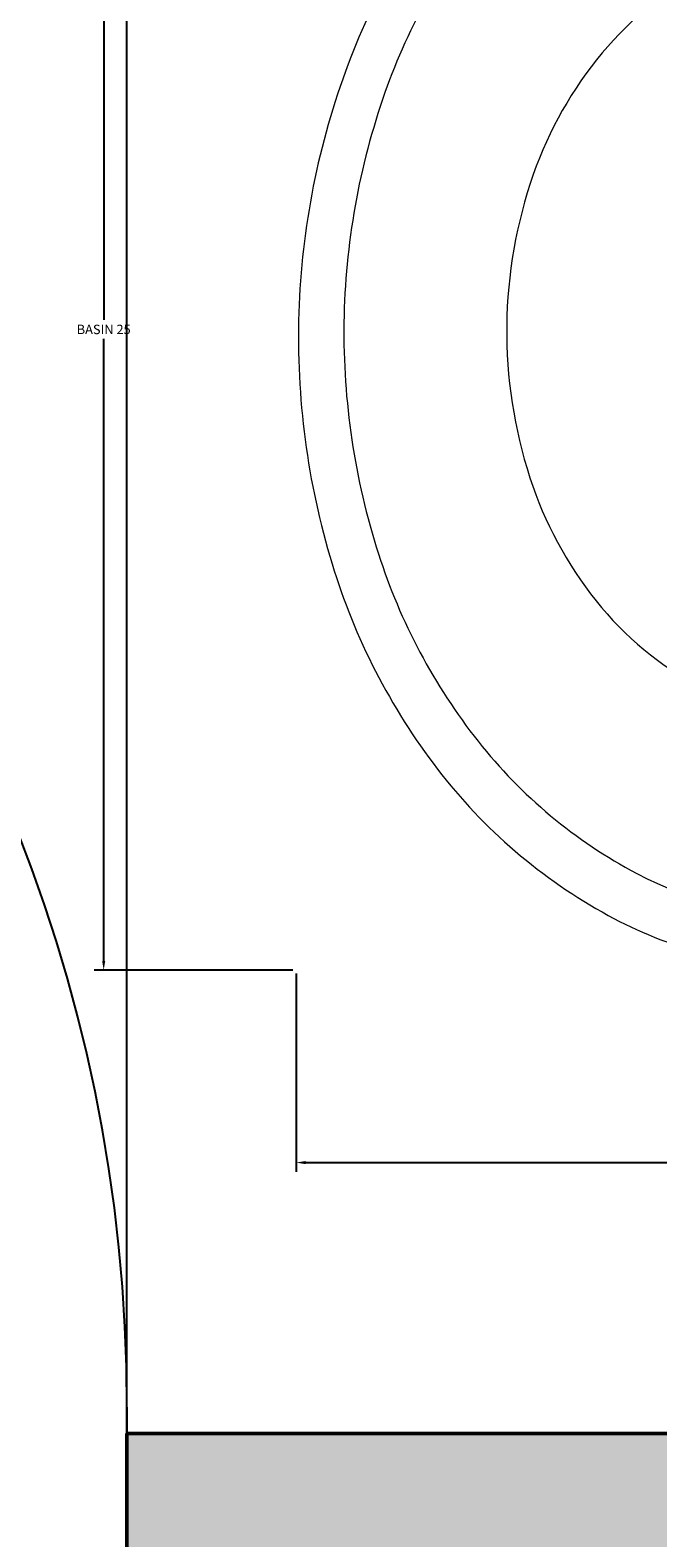
# Model space of a CAD drawing. Units: inches. Extents: x 2307 to 2544, y 2171 to 2540.
# Tile 41 of 52: x 2490 to 2502, y 2438 to 2466. Entities that reach past the tile are written whole.
import ezdxf

# ---------------------------------------------------------------- set-up
doc = ezdxf.new("R2010")
doc.units = ezdxf.units.IN
for name, color, linetype, lineweight in [('A-ANNO-DIMS', 2, 'Continuous', 18), ('A-DOOR', 3, 'Continuous', 25), ('A-FLOR-FIXT', 9, 'Continuous', 18), ('A-WALL', 7, 'Continuous', 50)]:
    doc.layers.add(name, color=color, linetype=linetype, lineweight=lineweight)
doc.layers.add('A-WALL-PATT', color=18, linetype='Continuous', lineweight=13, true_color=0x000000)
doc.styles.get("Standard").update_dxf_attribs({"font": 'arial.ttf'})
doc.dimstyles.get("Standard").update_dxf_attribs({"dimtxt": 0.18, "dimasz": 0.18, "dimexe": 0.18, "dimexo": 0.0625, "dimgap": 0.09, "dimtad": 0, "dimtih": 1, "dimtoh": 1, "dimdec": 4, "dimzin": 0, "dimdsep": 46, "dimtxsty": 'Standard', "dimcen": 0.09, "dimadec": 0, "dimazin": 0, "dimtfac": 1, "dimtdec": 4, "dimtofl": 0, "dimtmove": 0, "dimatfit": 3, "dimfxl": 1, "dimtolj": 1, "dimtzin": 0, "dimarcsym": 0})

# ---------------------------------------------------------------- blocks, each defined once
blk = doc.blocks.new('Sink - Oval top')
for p, q in [((0, 1), (0, -1)), ((-1, 0), (1, 0))]:
    blk.add_line(p, q)
for points in [[(-12.234, 0.394, 0.117634), (-11.465, -3.362, 0.104469), (-8.879, -6.804, 0.090016), (-5.083, -9.072, 0.08192), (-0.323, -10.016, 0.08192), (4.488, -9.381, 0.090016), (8.422, -7.361, 0.104469), (11.224, -4.093, 0.117634), (12.234, -0.394, 0.117634), (11.465, 3.362, 0.104469), (8.879, 6.804, 0.090016), (5.083, 9.072, 0.08192), (0.323, 10.016, 0.08192), (-4.488, 9.381, 0.090016), (-8.422, 7.361, 0.104469), (-11.224, 4.093, 0.117634)], [(-11.286, 0.159, 0.118622), (-10.516, -3.253, 0.104678), (-8.072, -6.359, 0.089562), (-4.538, -8.367, 0.081185), (-0.129, -9.152, 0.081185), (4.3, -8.492, 0.089562), (7.889, -6.584, 0.104678), (10.42, -3.548, 0.118622), (11.286, -0.159, 0.118622), (10.516, 3.253, 0.104678), (8.072, 6.359, 0.089562), (4.538, 8.367, 0.081185), (0.129, 9.152, 0.081185), (-4.3, 8.492, 0.089562), (-7.889, 6.584, 0.104678), (-10.42, 3.548, 0.118622)], [(-7.42, 0.083, 0.118283), (-6.907, -2.167, 0.104607), (-5.295, -4.21, 0.089718), (-2.967, -5.528, 0.081436), (-0.068, -6.037, 0.081436), (2.842, -5.593, 0.089718), (5.199, -4.327, 0.104607), (6.857, -2.321, 0.118283), (7.42, -0.083, 0.118283), (6.907, 2.167, 0.104607), (5.295, 4.21, 0.089718), (2.967, 5.528, 0.081436), (0.068, 6.037, 0.081436), (-2.842, 5.593, 0.089718), (-5.199, 4.327, 0.104607), (-6.857, 2.321, 0.118283)]]:
    blk.add_lwpolyline(points, format="xyb", close=True)
for radius in [1.5, 1]:
    blk.add_circle((0, 0), radius)
blk = doc.blocks.new('*U13')
blk.add_line((40, 0), (40, -6))
blk.add_arc((0, 0), 40, 0, 90)
blk = doc.blocks.new('*D22')
at = {"layer": 'A-ANNO-DIMS', "color": 0, "lineweight": -2, "transparency": 16777216}
for p, q in [((2494.871, 2472.93), (2491.071, 2472.93)), ((2491.251, 2472.75), (2491.251, 2460.838)), ((2491.251, 2448.56), (2491.251, 2460.472)), ((2494.871, 2448.38), (2491.071, 2448.38))]:
    blk.add_line(p, q, dxfattribs=at)
at = {"layer": 'A-ANNO-DIMS', "color": 0, "transparency": 16777216}
for points in [[(2491.221, 2472.75), (2491.281, 2472.75), (2491.251, 2472.93)], [(2491.221, 2448.56), (2491.281, 2448.56), (2491.251, 2448.38)]]:
    blk.add_solid(points, dxfattribs=at)
at = {"layer": 'Defpoints', "color": 0, "transparency": 16777216}
for p in [(2494.934, 2472.93), (2491.251, 2448.38), (2494.934, 2448.38)]:
    blk.add_point(p, dxfattribs=at)
at = {"layer": 'A-ANNO-DIMS', "color": 0, "transparency": 16777216, "insert": (2491.251, 2460.655), "char_height": 0.18, "attachment_point": 5}
blk.add_mtext('\\A1;BASIN 25', dxfattribs=at)
blk = doc.blocks.new('*D23')
at = {"layer": 'A-ANNO-DIMS', "color": 0, "lineweight": -2, "transparency": 16777216}
for p, q in [((2494.934, 2448.317), (2494.934, 2444.517)), ((2515.07, 2448.317), (2515.07, 2444.517)), ((2495.114, 2444.697), (2504.782, 2444.697)), ((2514.89, 2444.697), (2505.222, 2444.697))]:
    blk.add_line(p, q, dxfattribs=at)
at = {"layer": 'A-ANNO-DIMS', "color": 0, "transparency": 16777216}
for points in [[(2495.114, 2444.727), (2495.114, 2444.667), (2494.934, 2444.697)], [(2514.89, 2444.727), (2514.89, 2444.667), (2515.07, 2444.697)]]:
    blk.add_solid(points, dxfattribs=at)
at = {"layer": 'Defpoints', "color": 0, "transparency": 16777216}
for p in [(2494.934, 2448.38), (2515.07, 2448.38), (2515.07, 2444.697)]:
    blk.add_point(p, dxfattribs=at)
at = {"layer": 'A-ANNO-DIMS', "color": 0, "transparency": 16777216, "insert": (2505.002, 2444.697), "char_height": 0.18, "attachment_point": 5}
blk.add_mtext('\\A1;20', dxfattribs=at)
blk = doc.blocks.new('*D61')
at = {"layer": 'A-ANNO-DIMS', "color": 0, "lineweight": -2, "transparency": 16777216}
for p, q in [((2491.696, 2435.572), (2491.696, 2540.345)), ((2515.696, 2435.572), (2515.696, 2540.345)), ((2491.876, 2540.165), (2503.476, 2540.165)), ((2515.516, 2540.165), (2503.916, 2540.165))]:
    blk.add_line(p, q, dxfattribs=at)
at = {"layer": 'A-ANNO-DIMS', "color": 0, "transparency": 16777216}
for points in [[(2491.876, 2540.195), (2491.876, 2540.135), (2491.696, 2540.165)], [(2515.516, 2540.195), (2515.516, 2540.135), (2515.696, 2540.165)]]:
    blk.add_solid(points, dxfattribs=at)
at = {"layer": 'Defpoints', "color": 0, "transparency": 16777216}
for p in [(2515.696, 2540.165), (2491.696, 2435.51), (2515.696, 2435.51)]:
    blk.add_point(p, dxfattribs=at)
at = {"layer": 'A-ANNO-DIMS', "color": 0, "transparency": 16777216, "insert": (2503.696, 2540.165), "char_height": 0.18, "attachment_point": 5}
blk.add_mtext('\\A1;24', dxfattribs=at)

msp = doc.modelspace()

# ---------------------------------------------------------------- hatches: boundary and pattern name
at = {"layer": 'A-WALL-PATT'}
h = msp.add_hatch(color=256, dxfattribs=at)
h.dxf.hatch_style = 1
h.paths.add_polyline_path([(2433.6935, 2199.5096), (2415.6423, 2199.5096), (2415.6423, 2190.5096), (2433.7832, 2190.5096)], flags=17)
h.paths.add_polyline_path([(2367.6423, 2199.5096), (2335.6958, 2199.5096), (2335.6958, 2307.3983), (2326.6958, 2307.3983), (2326.6958, 2190.5096), (2367.6423, 2190.5096)])
h.paths.add_polyline_path([(2524.6958, 2520.5096), (2496.7832, 2520.5096), (2496.7832, 2515.5149), (2472.7832, 2515.5149), (2472.7832, 2520.5096), (2415.4028, 2520.5096), (2415.4028, 2511.5096), (2451.6958, 2511.5096), (2451.6958, 2439.5096), (2451.6958, 2391.5096), (2445.6958, 2391.5096), (2445.6958, 2387.5096), (2455.6958, 2387.5096), (2455.6958, 2435.5096), (2461.6958, 2435.5096), (2461.6958, 2439.5096), (2455.6958, 2439.5096), (2455.6958, 2511.5096), (2515.6958, 2511.5096), (2515.6958, 2439.5096), (2491.6958, 2439.5096), (2491.6958, 2435.5096), (2515.6958, 2435.5096), (2515.6958, 2319.5096), (2451.6958, 2319.5096), (2451.6958, 2281.5096), (2481.6958, 2281.5096), (2481.6958, 2225.5096), (2485.6958, 2225.5096), (2485.6958, 2285.5096), (2455.6958, 2285.5096), (2455.6958, 2315.5096), (2515.6958, 2315.5096), (2515.6958, 2199.5096), (2469.6952, 2199.5096), (2469.785, 2190.5096), (2524.6958, 2190.5096)])

# ---------------------------------------------------------------- linework, layer by layer
at = {"layer": 'A-WALL'}
for q in [(2491.6958, 2435.5096), (2515.6958, 2439.5096)]:
    msp.add_line((2491.6958, 2439.5096), q, dxfattribs=at)

# ---------------------------------------------------------------- block references
at = {"layer": 'A-DOOR', "xscale": 0.75, "yscale": 0.75, "zscale": 0.75}
msp.add_blockref('*U13', (2461.6958, 2440.0096), dxfattribs=at)
at = {"layer": 'A-FLOR-FIXT', "rotation": 270}
msp.add_blockref('Sink - Oval top', (2505.002, 2460.655), dxfattribs=at)

# ---------------------------------------------------------------- dimensions: what is measured, and where the dimension line sits
at = {"layer": 'A-ANNO-DIMS'}
for base, p1, p2, picture, middle in [((2515.6958, 2540.1649), (2491.6958, 2435.5096), (2515.6958, 2435.5096), '*D61', (2503.6958, 2540.1649)), ((2515.0703, 2444.6969), (2494.9337, 2448.3795), (2515.0703, 2448.3795), '*D23', (2505.002, 2444.6969))]:
    dim = msp.add_linear_dim(base=base, p1=p1, p2=p2, dimstyle='Standard', override={"dimdec": 0, "dimlfac": 1, "dimrnd": 0, "dimzin": 0, "dimdsep": 46, "dimlunit": 2}, dxfattribs=at)
    dim.commit()
    dim.dimension.update_dxf_attribs({"geometry": picture, "text_midpoint": middle})
dim = msp.add_linear_dim(base=(2491.2511, 2448.3795), p1=(2494.9337, 2472.9304), p2=(2494.9337, 2448.3795), angle=270, text='BASIN <>', dimstyle='Standard', override={"dimdec": 0, "dimlfac": 1, "dimrnd": 0, "dimzin": 0, "dimdsep": 46, "dimlunit": 2}, dxfattribs=at)
dim.commit()
dim.dimension.update_dxf_attribs({"geometry": '*D22', "text_midpoint": (2491.2511, 2460.655)})

doc.saveas('drawing.dxf')
